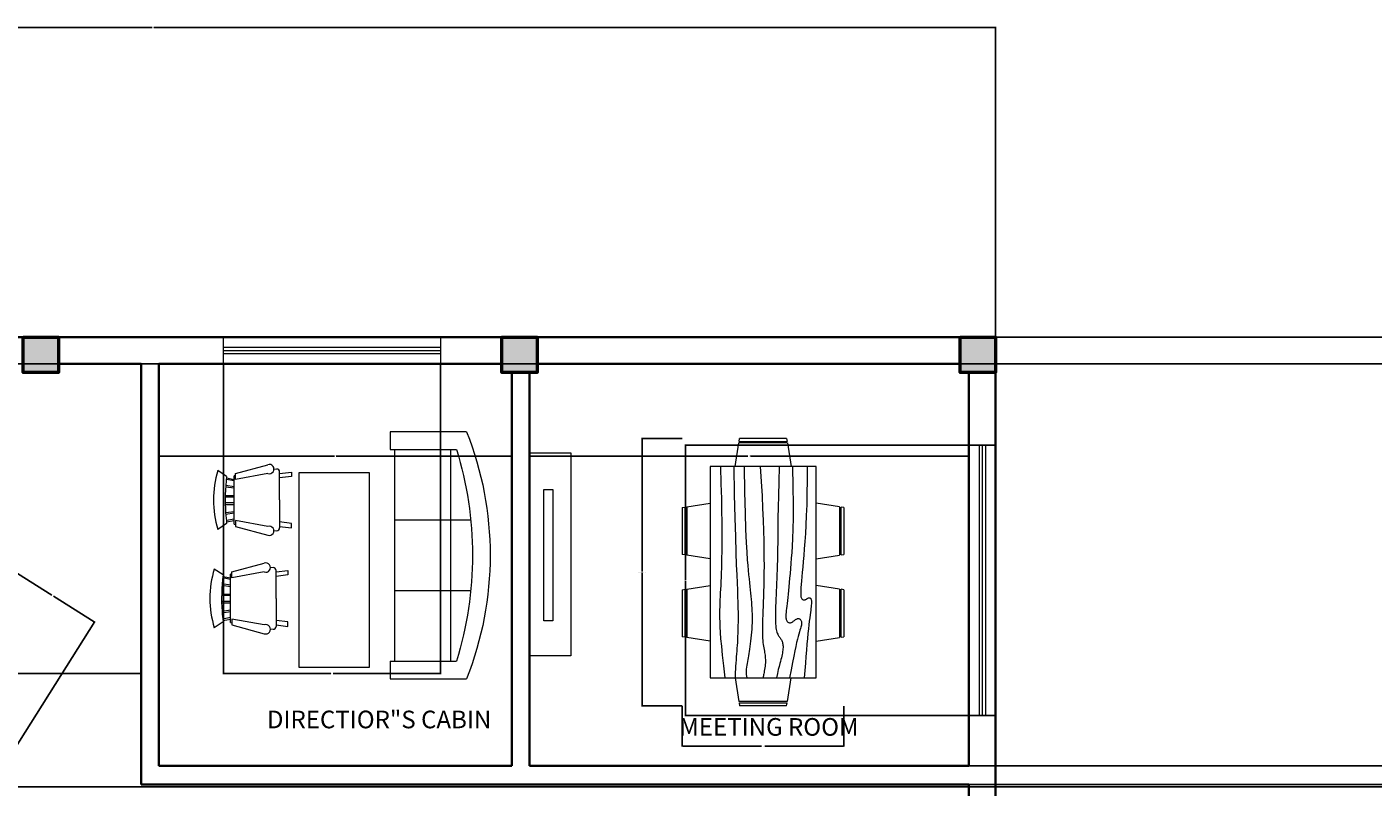
# Model space of a CAD drawing. Units: inches. Extents: x 369 to 4994, y 516 to 1297.
# Tile 6 of 9: x 1452 to 1910, y 886 to 1144. Entities that reach past the tile are written whole.
import ezdxf

# ---------------------------------------------------------------- set-up
doc = ezdxf.new("R2010")
doc.units = ezdxf.units.IN
doc.header["$MEASUREMENT"] = 0
for name, color, linetype, lineweight in [('A-ANNO-DIMS', 2, 'Continuous', 18), ('A-AREA-IDEN', 7, 'Continuous', 18), ('A-COLS', 7, 'Continuous', 50), ('A-FURN', 8, 'Continuous', 18), ('A-GLAZ', 4, 'Continuous', 18), ('A-WALL', 7, 'Continuous', 35)]:
    doc.layers.add(name, color=color, linetype=linetype, lineweight=lineweight)
doc.layers.add('A-COLS-PATT', color=18, linetype='Continuous', lineweight=13, true_color=0x000000)
doc.styles.get("Standard").update_dxf_attribs({"font": 'arial.ttf'})
doc.dimstyles.get("Standard").update_dxf_attribs({"dimtxt": 0.18, "dimasz": 0.18, "dimexe": 0.18, "dimexo": 0.0625, "dimgap": 0.09, "dimtad": 0, "dimtih": 1, "dimtoh": 1, "dimdec": 4, "dimzin": 0, "dimdsep": 46, "dimtxsty": 'Standard', "dimcen": 0.09, "dimadec": 0, "dimazin": 0, "dimtfac": 1, "dimtdec": 4, "dimtofl": 0, "dimtmove": 0, "dimatfit": 3, "dimfxl": 1, "dimtolj": 1, "dimtzin": 0, "dimarcsym": 0})

# ---------------------------------------------------------------- blocks, each defined once
blk = doc.blocks.new('Dining Set - 36 x 72 in.')
for p, q in [((-22, 27.5), (-22.1562, 26.50042)), ((-22, 27.5), (-6, 27.5)), ((-5.8437, 26.49966), (-6, 27.5)), ((6, 27.5), (5.8438, 26.50042)), ((6, 27.5), (22, 27.5)), ((22.1563, 26.49966), (22, 27.5)), ((-22.2343, 26.00059), (-23.4847, 17.99762)), ((-22.2304, 26), (-5.7608, 26)), ((-5.8416, 26.5), (-22.1534, 26.5)), ((-4.5152, 17.99762), (-5.7655, 25.99926)), ((5.7657, 26.00059), (4.5153, 17.99762)), ((5.7696, 26), (22.2392, 26)), ((22.1584, 26.5), (5.8466, 26.5)), ((23.4848, 17.99762), (22.2345, 25.99926)), ((36, 18), (-36, 18)), ((-36, 18), (-36, -18)), ((36, -18), (36, 18)), ((-44.0006, 8.23428), (-35.9976, 9.48474)), ((44.0006, 8.23428), (35.9976, 9.48474)), ((-45.5, 8), (-44.5004, 8.15617)), ((-45.5, 8), (-45.5, -8)), ((-44.5, -8.15843), (-44.5, 8.15338)), ((-44, 8.23041), (-44, -8.23915)), ((44, 8.23041), (44, -8.23915)), ((44.5, -8.15843), (44.5, 8.15338)), ((45.5, 8), (44.5005, 8.15617)), ((45.5, 8), (45.5, -8)), ((-44.4997, -8.15631), (-45.5, -8)), ((-35.9976, -9.48476), (-43.9993, -8.2345)), ((35.9976, -9.48476), (43.9993, -8.2345)), ((44.4997, -8.15631), (45.5, -8)), ((-36, -18), (36, -18)), ((-22.2343, -26.0006), (-23.4847, -17.99762)), ((-4.5152, -17.99762), (-5.7655, -25.99928)), ((5.7657, -26.0006), (4.5153, -17.99762)), ((23.4848, -17.99762), (22.2345, -25.99928)), ((-22.2304, -26), (-5.7608, -26)), ((-22, -27.5), (-22.1562, -26.50044)), ((-5.8416, -26.5), (-22.1534, -26.5)), ((-5.8437, -26.49967), (-6, -27.5)), ((5.7696, -26), (22.2392, -26)), ((6, -27.5), (5.8438, -26.50044)), ((22.1584, -26.5), (5.8466, -26.5)), ((22.1563, -26.49967), (22, -27.5)), ((-22, -27.5), (-6, -27.5)), ((6, -27.5), (22, -27.5))]:
    blk.add_line(p, q)
for points in [[(-36, 15), (-31.1772, 14.97754), (-26.8079, 14.91406), (-22.8538, 14.81543), (-19.276, 14.6875), (-16.0362, 14.53613), (-13.0957, 14.36718), (-10.4159, 14.18652), (-7.9583, 14), (-5.6904, 13.81315), (-3.6035, 13.63021), (-1.6954, 13.45508), (0.0365, 13.29166), (1.5945, 13.14388), (2.9811, 13.01562), (4.1988, 12.9108), (5.25, 12.83333), (6.1393, 12.78613), (6.8802, 12.76823), (7.4883, 12.77767), (7.9792, 12.8125), (8.3685, 12.87077), (8.6719, 12.95052), (8.9049, 13.0498), (9.0833, 13.16666), (9.2205, 13.29899), (9.3216, 13.44401), (9.3895, 13.59879), (9.4271, 13.76041), (9.4373, 13.92594), (9.4232, 14.09245), (9.3875, 14.257), (9.3333, 14.41666), (9.2638, 14.56917), (9.1836, 14.71484), (9.0975, 14.85465), (9.0104, 14.98958), (8.9272, 15.1206), (8.8529, 15.2487), (8.7922, 15.37483), (8.75, 15.5), (8.7305, 15.62467), (8.7344, 15.74739), (8.7617, 15.86621), (8.8125, 15.97916), (8.8867, 16.08431), (8.9844, 16.17968), (9.1055, 16.26334), (9.25, 16.33333), (9.4189, 16.38802), (9.6172, 16.42708), (9.8506, 16.45052), (10.125, 16.45833), (10.4463, 16.45052), (10.8203, 16.42708), (11.2529, 16.38802), (11.75, 16.33333), (12.3184, 16.26318), (12.9694, 16.17838), (13.7151, 16.07991), (14.5677, 15.96875), (15.5395, 15.84586), (16.6426, 15.71224), (17.8893, 15.56884), (19.2917, 15.41666), (20.859, 15.25667), (22.5879, 15.08984), (24.4721, 14.91715), (26.5052, 14.73958), (28.6809, 14.5581), (30.9929, 14.3737), (33.4347, 14.18733), (36, 14)], [(-36, 10), (-28.9766, 10.14274), (-23.1725, 10.20442), (-18.4241, 10.19775), (-14.5677, 10.13541), (-11.4399, 10.03011), (-8.877, 9.89453), (-6.7154, 9.74137), (-4.7917, 9.58333), (-2.9698, 9.43082), (-1.2246, 9.28515), (0.4415, 9.14534), (2.026, 9.01041), (3.5266, 8.87939), (4.9408, 8.7513), (6.266, 8.62516), (7.5, 8.5), (8.6411, 8.37549), (9.6914, 8.2539), (10.6538, 8.13818), (11.5312, 8.03125), (12.3267, 7.93603), (13.043, 7.85547), (13.6831, 7.79248), (14.25, 7.75), (14.7471, 7.7303), (15.1797, 7.73307), (15.5537, 7.75732), (15.875, 7.80208), (16.1494, 7.86637), (16.3828, 7.94922), (16.5811, 8.04964), (16.75, 8.16666), (16.8944, 8.29915), (17.0143, 8.44531), (17.1089, 8.60319), (17.1771, 8.77083), (17.218, 8.94629), (17.2305, 9.1276), (17.2137, 9.31282), (17.1667, 9.5), (17.0895, 9.6875), (16.987, 9.875), (16.8649, 10.0625), (16.7292, 10.25), (16.5856, 10.4375), (16.4401, 10.625), (16.2985, 10.8125), (16.1667, 11), (16.05, 11.18733), (15.9518, 11.3737), (15.8752, 11.5581), (15.8229, 11.73958), (15.798, 11.91715), (15.8034, 12.08984), (15.842, 12.25667), (15.9167, 12.41666), (16.0295, 12.56836), (16.1784, 12.70833), (16.3605, 12.83268), (16.5729, 12.9375), (16.8127, 13.01888), (17.0768, 13.07291), (17.3625, 13.0957), (17.6667, 13.08333), (17.9894, 13.03312), (18.3418, 12.94726), (18.7382, 12.82918), (19.1927, 12.68229), (19.7195, 12.51001), (20.3327, 12.31575), (21.0465, 12.10294), (21.875, 11.875), (22.8357, 11.63354), (23.959, 11.37304), (25.2786, 11.08618), (26.8282, 10.76562), (28.6414, 10.40405), (30.752, 9.99414), (33.1936, 9.52856), (36, 9)], [(-36, 5.5), (-30.7157, 5.3348), (-26.069, 5.20963), (-21.9946, 5.11767), (-18.4271, 5.05208), (-15.3009, 5.00602), (-12.5508, 4.97265), (-10.1112, 4.94515), (-7.9167, 4.91666), (-5.909, 4.88167), (-4.0586, 4.83984), (-2.3429, 4.79215), (-0.7396, 4.73958), (0.7739, 4.6831), (2.22, 4.6237), (3.6213, 4.56233), (5, 4.5), (6.373, 4.43782), (7.7344, 4.3776), (9.0723, 4.32129), (10.375, 4.27083), (11.6309, 4.22819), (12.8281, 4.19531), (13.9551, 4.17415), (15, 4.16666), (15.954, 4.17448), (16.819, 4.19791), (17.6001, 4.23698), (18.3021, 4.29166), (18.9299, 4.36198), (19.4883, 4.44791), (19.9823, 4.54948), (20.4167, 4.66666), (20.7969, 4.79899), (21.1302, 4.94401), (21.4245, 5.09879), (21.6875, 5.26041), (21.9271, 5.42594), (22.1511, 5.59245), (22.3672, 5.757), (22.5834, 5.91666), (22.8065, 6.06868), (23.0404, 6.21093), (23.2879, 6.34147), (23.5521, 6.45833), (23.8358, 6.55957), (24.142, 6.64323), (24.4735, 6.70735), (24.8334, 6.75), (25.2235, 6.76969), (25.642, 6.76692), (26.0858, 6.74267), (26.5521, 6.69791), (27.0379, 6.63362), (27.5404, 6.55078), (28.0565, 6.45036), (28.5834, 6.33333), (29.1242, 6.19987), (29.7071, 6.04687), (30.3661, 5.87044), (31.1354, 5.66666), (32.0493, 5.43164), (33.142, 5.16146), (34.4475, 4.85221), (36, 4.5)], [(-36, -1), (-30.7915, -0.6591), (-26.0195, -0.38216), (-21.6519, -0.16284), (-17.6563, 0.00521), (-14.0005, 0.12833), (-10.6523, 0.21289), (-7.5796, 0.26522), (-4.75, 0.29166), (-2.134, 0.29793), (0.2878, 0.28711), (2.5317, 0.26163), (4.6146, 0.22396), (6.5529, 0.17651), (8.3633, 0.12174), (10.0623, 0.06209), (11.6667, 0), (13.1899, -0.06201), (14.6341, -0.1211), (15.9982, -0.17432), (17.2813, -0.21875), (18.4823, -0.25147), (19.6003, -0.26953), (20.6343, -0.27002), (21.5834, -0.25), (22.4481, -0.20768), (23.2357, -0.14584), (23.9549, -0.06836), (24.6146, 0.02083), (25.2235, 0.11784), (25.7904, 0.21875), (26.3241, 0.31966), (26.8334, 0.41666), (27.3265, 0.50618), (27.8099, 0.58593), (28.2894, 0.65397), (28.7709, 0.70833), (29.2601, 0.74707), (29.763, 0.76823), (30.2855, 0.76985), (30.8334, 0.75), (31.4088, 0.70784), (31.9994, 0.64713), (32.589, 0.57275), (33.1615, 0.48958), (33.7008, 0.4025), (34.1908, 0.3164), (34.6153, 0.23616), (34.9584, 0.16666), (35.2099, 0.11165), (35.3848, 0.07031), (35.504, 0.04069), (35.5886, 0.02083), (35.6594, 0.00879), (35.7377, 0.0026), (35.8442, 0.00032), (36, 0)], [(-36, -6.5), (-27.1843, -6.31267), (-20.084, -6.1263), (-14.469, -5.9419), (-10.1094, -5.76042), (-6.7752, -5.58285), (-4.2363, -5.41016), (-2.2629, -5.24333), (-0.625, -5.08334), (0.8708, -4.93099), (2.2715, -4.78646), (3.5872, -4.64974), (4.8281, -4.52084), (6.0046, -4.39974), (7.127, -4.28646), (8.2053, -4.18099), (9.25, -4.08334), (10.2705, -3.99382), (11.2734, -3.91407), (12.2647, -3.84603), (13.25, -3.79167), (14.2354, -3.75293), (15.2266, -3.73177), (16.2295, -3.73015), (17.25, -3.75), (18.2912, -3.79248), (19.3451, -3.85547), (20.4009, -3.93604), (21.4479, -4.03125), (22.4754, -4.13819), (23.4727, -4.25391), (24.4289, -4.37549), (25.3334, -4.5), (26.1785, -4.62492), (26.9694, -4.74935), (27.7145, -4.87281), (28.4219, -4.99479), (29.1, -5.11483), (29.7572, -5.23242), (30.4016, -5.34709), (31.0417, -5.45834), (31.6837, -5.56437), (32.3262, -5.65821), (32.9658, -5.73153), (33.599, -5.77604), (34.2224, -5.78345), (34.8327, -5.74545), (35.4264, -5.65373), (36, -5.5)], [(-36, -10), (-26.4022, -9.81299), (-18.4675, -9.62891), (-11.9839, -9.45069), (-6.7396, -9.28125), (-2.5226, -9.12354), (0.8789, -8.98047), (3.6769, -8.85498), (6.0833, -8.75), (8.2767, -8.66765), (10.3021, -8.60677), (12.1712, -8.56543), (13.8958, -8.54167), (15.4876, -8.53353), (16.9583, -8.53907), (18.3197, -8.55632), (19.5834, -8.58334), (20.7616, -8.61841), (21.8685, -8.66081), (22.9188, -8.71004), (23.9271, -8.76563), (24.9081, -8.82707), (25.8763, -8.89388), (26.8465, -8.96558), (27.8334, -9.04167), (28.8474, -9.12118), (29.8828, -9.20117), (30.93, -9.27824), (31.9792, -9.34896), (33.0205, -9.40991), (34.0443, -9.45768), (35.0407, -9.48885), (36, -9.5)], [(-36, -14.5), (-30.0881, -14.33513), (-25.0332, -14.21224), (-20.7312, -14.12647), (-17.0781, -14.07292), (-13.97, -14.04671), (-11.3027, -14.04297), (-8.9724, -14.05681), (-6.875, -14.08334), (-4.9224, -14.11833), (-3.0905, -14.16016), (-1.3709, -14.20785), (0.2448, -14.26042), (1.7647, -14.3169), (3.1973, -14.3763), (4.5507, -14.43767), (5.8333, -14.5), (7.0554, -14.5621), (8.235, -14.62175), (9.3922, -14.67652), (10.5469, -14.72396), (11.7192, -14.76164), (12.929, -14.78711), (14.1965, -14.79794), (15.5417, -14.79167), (16.9933, -14.76424), (18.6152, -14.70508), (20.4804, -14.60197), (22.6615, -14.44271), (25.2312, -14.21509), (28.2624, -13.9069), (31.8277, -13.50594), (36, -13)]]:
    blk.add_lwpolyline(points)
blk = doc.blocks.new('Chair - Rocking')
for p, q in [((-8, -4.5), (-10, -1.5)), ((-7.5, -4.5), (-7, -7)), ((-6.5, -7), (-7.02225, -4.43)), ((-4.5, -7), (-4.96674, -4.19951)), ((-4, -7), (-4.40532, -4.16272)), ((-1.5, -4.05012), (-1.5, -7)), ((-1, -7), (-1, -4.05012)), ((1, -7), (1, -4.04655)), ((1.5, -4.05012), (1.5, -7)), ((4, -7), (4.40187, -4.18694)), ((4.5, -7), (4.96761, -4.19437)), ((6.5, -7), (7, -4.4057)), ((7.5, -4.5), (7, -7)), ((8, -4.5), (10, -1.5)), ((-9, -7.5), (-12, -18.49999)), ((-7, -7.5), (-9, -7.5)), ((-9, -18.49999), (-7, -7.5)), ((-8.23428, -6.99939), (-8.3093, -7.47958)), ((-8.23041, -7), (8.23915, -7)), ((7, -7.5), (9, -7.5)), ((9, -18.49999), (7, -7.5)), ((8.31071, -7.48854), (8.23449, -7.00073)), ((9, -7.5), (12, -18.49999)), ((-10.36644, -20.64523), (-10.5, -21.49999)), ((-9, -22.49999), (-9.5, -26.49999)), ((0, -22.49999), (-9.5, -22.49999)), ((-8, -26.49999), (-7.5, -22.49999)), ((0, -22.49999), (9.5, -22.49999)), ((8, -26.49999), (7.5, -22.49999)), ((9, -22.49999), (9.5, -26.49999)), ((10.5, -21.49999), (10.3575, -20.58798)), ((-9.5, -26.49999), (-8, -26.49999)), ((9.5, -26.49999), (8, -26.49999))]:
    blk.add_line(p, q)
for centre, radius, start, end in [((0, -34.08333), 34.08333, 72.93847, 107.0615), ((0, -68.25004), 64.25, 93.92211, 97.15267), ((0, -68.25004), 64.25, 82.84733, 93.92211), ((-10.5, -18.99999), 1.58114, 161.5651, 18.43495), ((-9.5, -21.49999), 1, 180, 270), ((10.5, -18.99999), 1.58114, 161.5651, 18.43495), ((9.5, -21.49999), 1, 270, 0)]:
    blk.add_arc(centre, radius, start, end)
blk = doc.blocks.new('Sofa - Roundback 7 ft.')
for p, q in [((-12.00002, -32.4421), (-12.00003, -6.5971)), ((11.99997, -32.4421), (11.99998, -6.5971)), ((-36.000027, -34), (-36.000027, -11.4696)), ((-35.999844, -13.3819), (35.9998, -13.3819)), ((35.99998, -34), (35.99998, -11.4696)), ((-36.000027, -32.4421), (35.99998, -32.4421))]:
    blk.add_line(p, q)
for points in [[(-36.000027, -34), (-42.000027, -34), (-42.000027, -8)], [(41.99998, -8), (41.99998, -34), (35.99998, -34)]]:
    blk.add_lwpolyline(points)
for centre, radius, start, end in [((0, -114.25), 114.25, 68.43141, 111.5686), ((-0.00001, -127.1968), 121.1968, 72.72033, 107.2797)]:
    blk.add_arc(centre, radius, start, end)
blk = doc.blocks.new('*D17')
at = {"layer": 'A-ANNO-DIMS', "color": 0, "lineweight": -2, "transparency": 16777216}
for p, q in [((1674.81, 1004.36), (1661.04, 1004.36)), ((1661.22, 1004.18), (1661.22, 959.05)), ((1661.22, 913.54), (1661.22, 958.68)), ((1674.81, 913.36), (1661.04, 913.36))]:
    blk.add_line(p, q, dxfattribs=at)
at = {"layer": 'A-ANNO-DIMS', "color": 0, "transparency": 16777216}
for points in [[(1661.19, 1004.18), (1661.25, 1004.18), (1661.22, 1004.36)], [(1661.19, 913.54), (1661.25, 913.54), (1661.22, 913.36)]]:
    blk.add_solid(points, dxfattribs=at)
at = {"layer": 'Defpoints', "color": 0, "transparency": 16777216}
for p in [(1674.87, 1004.36), (1661.22, 913.36), (1674.87, 913.36)]:
    blk.add_point(p, dxfattribs=at)
at = {"layer": 'A-ANNO-DIMS', "color": 0, "transparency": 16777216, "insert": (1661.22, 958.86), "char_height": 0.18, "attachment_point": 5}
blk.add_mtext('\\A1;TABLE & CHAIRS 91 TYP.', dxfattribs=at)
blk = doc.blocks.new('*D18')
at = {"layer": 'A-ANNO-DIMS', "color": 0, "lineweight": -2, "transparency": 16777216}
for p, q in [((1674.87, 913.3), (1674.87, 899.53)), ((1729.87, 913.3), (1729.87, 899.53)), ((1675.05, 899.71), (1701.84, 899.71)), ((1729.69, 899.71), (1702.9, 899.71))]:
    blk.add_line(p, q, dxfattribs=at)
at = {"layer": 'A-ANNO-DIMS', "color": 0, "transparency": 16777216}
for points in [[(1675.05, 899.74), (1675.05, 899.68), (1674.87, 899.71)], [(1729.69, 899.74), (1729.69, 899.68), (1729.87, 899.71)]]:
    blk.add_solid(points, dxfattribs=at)
at = {"layer": 'Defpoints', "color": 0, "transparency": 16777216}
for p in [(1674.87, 913.36), (1729.87, 913.36), (1729.87, 899.71)]:
    blk.add_point(p, dxfattribs=at)
at = {"layer": 'A-ANNO-DIMS', "color": 0, "transparency": 16777216, "insert": (1702.37, 899.71), "char_height": 0.18, "attachment_point": 5}
blk.add_mtext('\\A1;55 TYP.', dxfattribs=at)
blk = doc.blocks.new('*D46')
at = {"layer": 'A-ANNO-DIMS', "color": 0, "lineweight": -2, "transparency": 16777216}
for p, q in [((978.32, 1029.79), (2671.51, 1029.79)), ((2671.33, 1029.61), (2671.33, 957.97)), ((2671.33, 885.97), (2671.33, 957.61)), ((1038.32, 885.79), (2671.51, 885.79))]:
    blk.add_line(p, q, dxfattribs=at)
at = {"layer": 'A-ANNO-DIMS', "color": 0, "transparency": 16777216}
for points in [[(2671.3, 1029.61), (2671.36, 1029.61), (2671.33, 1029.79)], [(2671.3, 885.97), (2671.36, 885.97), (2671.33, 885.79)]]:
    blk.add_solid(points, dxfattribs=at)
at = {"layer": 'Defpoints', "color": 0, "transparency": 16777216}
for p in [(978.26, 1029.79), (2671.33, 1029.79), (1038.26, 885.79)]:
    blk.add_point(p, dxfattribs=at)
at = {"layer": 'A-ANNO-DIMS', "color": 0, "transparency": 16777216, "insert": (2671.33, 957.79), "char_height": 0.18, "attachment_point": 5}
blk.add_mtext('\\A1;144', dxfattribs=at)
blk = doc.blocks.new('*D74')
at = {"layer": 'A-ANNO-DIMS', "color": 0, "lineweight": -2, "transparency": 16777216}
for p, q in [((1208.37, 1038.85), (1208.37, 1144.37)), ((1208.55, 1144.19), (1494.58, 1144.19)), ((1781.19, 1144.19), (1495.16, 1144.19)), ((1781.37, 1038.85), (1781.37, 1144.37))]:
    blk.add_line(p, q, dxfattribs=at)
at = {"layer": 'A-ANNO-DIMS', "color": 0, "transparency": 16777216}
for points in [[(1208.55, 1144.22), (1208.55, 1144.16), (1208.37, 1144.19)], [(1781.19, 1144.22), (1781.19, 1144.16), (1781.37, 1144.19)]]:
    blk.add_solid(points, dxfattribs=at)
at = {"layer": 'Defpoints', "color": 0, "transparency": 16777216}
for p in [(1781.37, 1144.19), (1208.37, 1038.79), (1781.37, 1038.79)]:
    blk.add_point(p, dxfattribs=at)
at = {"layer": 'A-ANNO-DIMS', "color": 0, "transparency": 16777216, "insert": (1494.87, 1144.19), "char_height": 0.18, "attachment_point": 5}
blk.add_mtext('\\A1;573', dxfattribs=at)
blk = doc.blocks.new('*D76')
at = {"layer": 'A-ANNO-DIMS', "color": 0, "lineweight": -2, "transparency": 16777216}
for p, q in [((1277.37, 1029.73), (1277.37, 924.21)), ((1490.89, 1029.73), (1490.89, 924.21)), ((1277.55, 924.39), (1383.74, 924.39)), ((1490.71, 924.39), (1384.53, 924.39))]:
    blk.add_line(p, q, dxfattribs=at)
at = {"layer": 'A-ANNO-DIMS', "color": 0, "transparency": 16777216}
for points in [[(1277.55, 924.42), (1277.55, 924.36), (1277.37, 924.39)], [(1490.71, 924.42), (1490.71, 924.36), (1490.89, 924.39)]]:
    blk.add_solid(points, dxfattribs=at)
at = {"layer": 'Defpoints', "color": 0, "transparency": 16777216}
for p in [(1277.37, 1029.79), (1490.89, 1029.79), (1277.37, 924.39)]:
    blk.add_point(p, dxfattribs=at)
at = {"layer": 'A-ANNO-DIMS', "color": 0, "transparency": 16777216, "insert": (1384.13, 924.39), "char_height": 0.18, "attachment_point": 5}
blk.add_mtext('\\A1;213.5', dxfattribs=at)
blk = doc.blocks.new('*D77')
at = {"layer": 'A-ANNO-DIMS', "color": 0, "lineweight": -2, "transparency": 16777216}
for p, q in [((1496.89, 893.03), (1496.89, 998.55)), ((1497.07, 998.37), (1556.61, 998.37)), ((1616.71, 998.37), (1557.17, 998.37)), ((1616.89, 893.03), (1616.89, 998.55))]:
    blk.add_line(p, q, dxfattribs=at)
at = {"layer": 'A-ANNO-DIMS', "color": 0, "transparency": 16777216}
for points in [[(1497.07, 998.4), (1497.07, 998.34), (1496.89, 998.37)], [(1616.71, 998.4), (1616.71, 998.34), (1616.89, 998.37)]]:
    blk.add_solid(points, dxfattribs=at)
at = {"layer": 'Defpoints', "color": 0, "transparency": 16777216}
for p in [(1616.89, 998.37), (1496.89, 892.97), (1616.89, 892.97)]:
    blk.add_point(p, dxfattribs=at)
at = {"layer": 'A-ANNO-DIMS', "color": 0, "transparency": 16777216, "insert": (1556.89, 998.37), "char_height": 0.18, "attachment_point": 5}
blk.add_mtext('\\A1;120', dxfattribs=at)
blk = doc.blocks.new('*D78')
at = {"layer": 'A-ANNO-DIMS', "color": 0, "lineweight": -2, "transparency": 16777216}
for p, q in [((1622.89, 893.03), (1622.89, 998.55)), ((1623.07, 998.37), (1697.18, 998.37)), ((1772.19, 998.37), (1698.09, 998.37)), ((1772.37, 893.03), (1772.37, 998.55))]:
    blk.add_line(p, q, dxfattribs=at)
at = {"layer": 'A-ANNO-DIMS', "color": 0, "transparency": 16777216}
for points in [[(1623.07, 998.4), (1623.07, 998.34), (1622.89, 998.37)], [(1772.19, 998.4), (1772.19, 998.34), (1772.37, 998.37)]]:
    blk.add_solid(points, dxfattribs=at)
at = {"layer": 'Defpoints', "color": 0, "transparency": 16777216}
for p in [(1772.37, 998.37), (1622.89, 892.97), (1772.37, 892.97)]:
    blk.add_point(p, dxfattribs=at)
at = {"layer": 'A-ANNO-DIMS', "color": 0, "transparency": 16777216, "insert": (1697.63, 998.37), "char_height": 0.18, "attachment_point": 5}
blk.add_mtext('\\A1;149.48', dxfattribs=at)
blk = doc.blocks.new('*D79')
at = {"layer": 'A-ANNO-DIMS', "color": 0, "lineweight": -2, "transparency": 16777216}
for p, q in [((1769.44, 1029.79), (2671.51, 1029.79)), ((2671.33, 1029.61), (2671.33, 961.56)), ((2671.33, 893.15), (2671.33, 961.2)), ((1772.44, 892.97), (2671.51, 892.97))]:
    blk.add_line(p, q, dxfattribs=at)
at = {"layer": 'A-ANNO-DIMS', "color": 0, "transparency": 16777216}
for points in [[(2671.3, 1029.61), (2671.36, 1029.61), (2671.33, 1029.79)], [(2671.3, 893.15), (2671.36, 893.15), (2671.33, 892.97)]]:
    blk.add_solid(points, dxfattribs=at)
at = {"layer": 'Defpoints', "color": 0, "transparency": 16777216}
for p in [(1769.37, 1029.79), (2671.33, 1029.79), (1772.37, 892.97)]:
    blk.add_point(p, dxfattribs=at)
at = {"layer": 'A-ANNO-DIMS', "color": 0, "transparency": 16777216, "insert": (2671.33, 961.38), "char_height": 0.18, "attachment_point": 5}
blk.add_mtext('\\A1;136.82', dxfattribs=at)
blk = doc.blocks.new('*D80')
at = {"layer": 'A-ANNO-DIMS', "color": 0, "lineweight": -2, "transparency": 16777216}
for p, q in [((1772.44, 886.6), (2671.51, 886.6)), ((2671.33, 886.42), (2671.33, 847.38)), ((2671.33, 807.97), (2671.33, 847.01)), ((1772.44, 807.79), (2671.51, 807.79))]:
    blk.add_line(p, q, dxfattribs=at)
at = {"layer": 'A-ANNO-DIMS', "color": 0, "transparency": 16777216}
for points in [[(2671.3, 886.42), (2671.36, 886.42), (2671.33, 886.6)], [(2671.3, 807.97), (2671.36, 807.97), (2671.33, 807.79)]]:
    blk.add_solid(points, dxfattribs=at)
at = {"layer": 'Defpoints', "color": 0, "transparency": 16777216}
for p in [(1772.37, 886.6), (2671.33, 886.6), (1772.37, 807.79)]:
    blk.add_point(p, dxfattribs=at)
at = {"layer": 'A-ANNO-DIMS', "color": 0, "transparency": 16777216, "insert": (2671.33, 847.19), "char_height": 0.18, "attachment_point": 5}
blk.add_mtext('\\A1;78.81', dxfattribs=at)
blk = doc.blocks.new('*D88')
at = {"layer": 'A-ANNO-DIMS', "color": 0, "lineweight": -2, "transparency": 16777216}
for p, q in [((1390.27, 870.84), (1446.63, 960.04)), ((1446.68, 959.8), (1460.49, 951.07)), ((1474.87, 941.99), (1461.06, 950.71)), ((1418.75, 852.84), (1475.12, 942.04))]:
    blk.add_line(p, q, dxfattribs=at)
at = {"layer": 'A-ANNO-DIMS', "color": 0, "transparency": 16777216}
for points in [[(1446.7, 959.82), (1446.67, 959.77), (1446.53, 959.89)], [(1474.88, 942.01), (1474.85, 941.96), (1475.02, 941.89)]]:
    blk.add_solid(points, dxfattribs=at)
at = {"layer": 'Defpoints', "color": 0, "transparency": 16777216}
for p in [(1475.02, 941.89), (1390.23, 870.79), (1418.72, 852.79)]:
    blk.add_point(p, dxfattribs=at)
at = {"layer": 'A-ANNO-DIMS', "color": 0, "transparency": 16777216, "insert": (1460.78, 950.89), "char_height": 0.18, "attachment_point": 5}
blk.add_mtext('\\A1;33.7', dxfattribs=at)
blk = doc.blocks.new('*D94')
at = {"layer": 'A-ANNO-DIMS', "color": 0, "lineweight": -2, "transparency": 16777216}
for p, q in [((1518.87, 1029.73), (1518.87, 924.21)), ((1592.65, 1029.73), (1592.65, 924.21)), ((1519.05, 924.39), (1555.37, 924.39)), ((1592.47, 924.39), (1556.15, 924.39))]:
    blk.add_line(p, q, dxfattribs=at)
at = {"layer": 'A-ANNO-DIMS', "color": 0, "transparency": 16777216}
for points in [[(1519.05, 924.42), (1519.05, 924.36), (1518.87, 924.39)], [(1592.47, 924.42), (1592.47, 924.36), (1592.65, 924.39)]]:
    blk.add_solid(points, dxfattribs=at)
at = {"layer": 'Defpoints', "color": 0, "transparency": 16777216}
for p in [(1518.87, 1029.79), (1592.65, 1029.79), (1518.87, 924.39)]:
    blk.add_point(p, dxfattribs=at)
at = {"layer": 'A-ANNO-DIMS', "color": 0, "transparency": 16777216, "insert": (1555.76, 924.39), "char_height": 0.18, "attachment_point": 5}
blk.add_mtext('\\A1;73.77', dxfattribs=at)
blk = doc.blocks.new('*D95')
at = {"layer": 'A-ANNO-DIMS', "color": 0, "lineweight": -2, "transparency": 16777216}
for p, q in [((1781.31, 1002.1), (1675.79, 1002.1)), ((1675.97, 1001.92), (1675.97, 956.27)), ((1675.97, 910.26), (1675.97, 955.91)), ((1781.31, 910.08), (1675.79, 910.08))]:
    blk.add_line(p, q, dxfattribs=at)
at = {"layer": 'A-ANNO-DIMS', "color": 0, "transparency": 16777216}
for points in [[(1675.94, 1001.92), (1676, 1001.92), (1675.97, 1002.1)], [(1675.94, 910.26), (1676, 910.26), (1675.97, 910.08)]]:
    blk.add_solid(points, dxfattribs=at)
at = {"layer": 'Defpoints', "color": 0, "transparency": 16777216}
for p in [(1675.97, 1002.1), (1781.37, 1002.1), (1781.37, 910.08)]:
    blk.add_point(p, dxfattribs=at)
at = {"layer": 'A-ANNO-DIMS', "color": 0, "transparency": 16777216, "insert": (1675.97, 956.09), "char_height": 0.18, "attachment_point": 5}
blk.add_mtext('\\A1;92.02', dxfattribs=at)
blk = doc.blocks.new('*D98')
at = {"layer": 'A-ANNO-DIMS', "color": 0, "lineweight": -2, "transparency": 16777216}
for p, q in [((1992.86, 1038.79), (368.68, 1038.79)), ((368.86, 1038.61), (368.86, 830.47)), ((368.86, 621.97), (368.86, 830.11)), ((2046.86, 621.79), (368.68, 621.79))]:
    blk.add_line(p, q, dxfattribs=at)
at = {"layer": 'A-ANNO-DIMS', "color": 0, "transparency": 16777216}
for points in [[(368.83, 1038.61), (368.89, 1038.61), (368.86, 1038.79)], [(368.83, 621.97), (368.89, 621.97), (368.86, 621.79)]]:
    blk.add_solid(points, dxfattribs=at)
at = {"layer": 'Defpoints', "color": 0, "transparency": 16777216}
for p in [(368.86, 1038.79), (1992.93, 1038.79), (2046.93, 621.79)]:
    blk.add_point(p, dxfattribs=at)
at = {"layer": 'A-ANNO-DIMS', "color": 0, "transparency": 16777216, "insert": (368.86, 830.29), "char_height": 0.18, "attachment_point": 5}
blk.add_mtext('\\A1;417', dxfattribs=at)

msp = doc.modelspace()

# ---------------------------------------------------------------- hatches: boundary and pattern name
at = {"layer": 'A-COLS-PATT'}
h = msp.add_hatch(color=256, dxfattribs=at)
h.dxf.hatch_style = 1
h.paths.add_polyline_path([(540.2581, 633.7894), (528.2581, 633.7894), (528.2581, 621.7894), (540.2581, 621.7894)])
h.paths.add_polyline_path([(726.2581, 633.7894), (714.2581, 633.7894), (714.2581, 621.7894), (726.2581, 621.7894)])
h.paths.add_polyline_path([(918.2581, 633.7894), (906.2581, 633.7894), (906.2581, 621.7894), (918.2581, 621.7894)])
h.paths.add_polyline_path([(1047.2581, 633.7894), (1035.2581, 633.7894), (1035.2581, 621.7894), (1047.2581, 621.7894)])
h.paths.add_polyline_path([(1047.2581, 798.6977), (1035.2581, 798.6977), (1035.2581, 786.6977), (1047.2581, 786.6977)])
h.paths.add_polyline_path([(918.2581, 795.7894), (906.2581, 795.7894), (906.2581, 783.7894), (918.2581, 783.7894)])
h.paths.add_polyline_path([(726.2581, 795.7894), (714.2581, 795.7894), (714.2581, 783.7894), (726.2581, 783.7894)])
h.paths.add_polyline_path([(1047.2581, 1038.7894), (1035.2581, 1038.7894), (1035.2581, 1026.7894), (1047.2581, 1026.7894)])
h.paths.add_polyline_path([(855.044, 1038.7894), (843.044, 1038.7894), (843.044, 1026.7894), (855.044, 1026.7894)])
h.paths.add_polyline_path([(728.5536, 1038.7894), (716.5536, 1038.7894), (716.5536, 1026.7894), (728.5536, 1026.7894)])
h.paths.add_polyline_path([(543.2581, 1038.7894), (531.2581, 1038.7894), (531.2581, 1026.7894), (543.2581, 1026.7894)])
h.paths.add_polyline_path([(543.2581, 792.9013), (531.2581, 792.9013), (531.2581, 780.9013), (543.2581, 780.9013), (543.2581, 783.7894)])
h.paths.add_polyline_path([(1274.3738, 633.7894), (1262.3738, 633.7894), (1262.3738, 621.7894), (1274.3738, 621.7894)])
h.paths.add_polyline_path([(1460.3738, 633.7894), (1448.3738, 633.7894), (1448.3738, 621.7894), (1460.3738, 621.7894)])
h.paths.add_polyline_path([(1652.3738, 633.7894), (1640.3738, 633.7894), (1640.3738, 621.7894), (1652.3738, 621.7894)])
h.paths.add_polyline_path([(1781.3738, 633.7894), (1769.3738, 633.7894), (1769.3738, 621.7894), (1781.3738, 621.7894)])
h.paths.add_polyline_path([(1781.3738, 1038.7894), (1769.3738, 1038.7894), (1769.3738, 1026.7894), (1781.3738, 1026.7894)])
h.paths.add_polyline_path([(1625.484, 1038.7894), (1613.484, 1038.7894), (1613.484, 1026.7894), (1615.6962, 1026.7894), (1625.484, 1026.7894)])
h.paths.add_polyline_path([(1462.6692, 1038.7894), (1450.6692, 1038.7894), (1450.6692, 1026.7894), (1462.6692, 1026.7894)])
h.paths.add_polyline_path([(1277.3738, 1038.7894), (1265.3738, 1038.7894), (1265.3738, 1026.7894), (1277.3738, 1026.7894)])
h.paths.add_polyline_path([(1460.3738, 807.7894), (1448.3738, 807.7894), (1448.3738, 795.7894), (1460.3738, 795.7894)])
h.paths.add_polyline_path([(1652.3738, 807.7894), (1640.3738, 807.7894), (1640.3738, 795.7894), (1652.3738, 795.7894)])
h.paths.add_polyline_path([(2244.9265, 633.7894), (2232.9265, 633.7894), (2232.9265, 621.7894), (2244.9265, 621.7894)])
h.paths.add_polyline_path([(2058.9265, 633.7894), (2046.9265, 633.7894), (2046.9265, 621.7894), (2058.9265, 621.7894)])
h.paths.add_polyline_path([(2436.9265, 633.7894), (2424.9265, 633.7894), (2424.9265, 621.7894), (2436.9265, 621.7894)])
h.paths.add_polyline_path([(2565.9265, 633.7894), (2553.9265, 633.7894), (2553.9265, 621.7894), (2565.9265, 621.7894)])
h.paths.add_polyline_path([(2565.9265, 798.6977), (2553.9265, 798.6977), (2553.9265, 786.6977), (2565.9265, 786.6977)])
h.paths.add_polyline_path([(2565.9265, 1038.7894), (2553.9265, 1038.7894), (2553.9265, 1026.7894), (2565.9265, 1026.7894)])
h.paths.add_polyline_path([(2436.9265, 1038.7894), (2424.9265, 1038.7894), (2424.9265, 1026.7894), (2436.9265, 1026.7894)])
h.paths.add_polyline_path([(2247.222, 1038.7894), (2235.222, 1038.7894), (2235.222, 1026.7894), (2247.222, 1026.7894)])
h.paths.add_polyline_path([(2061.9265, 1038.7894), (2049.9265, 1038.7894), (2049.9265, 1026.7894), (2061.9265, 1026.7894)])

# ---------------------------------------------------------------- linework, layer by layer
at = {"layer": 'A-COLS'}
for points in [[(1450.6692, 1038.7894), (1462.6692, 1038.7894), (1462.6692, 1026.7894), (1450.6692, 1026.7894)], [(1769.3738, 1038.7894), (1781.3738, 1038.7894), (1781.3738, 1026.7894), (1769.3738, 1026.7894)]]:
    msp.add_lwpolyline(points, close=True, dxfattribs=at)
msp.add_lwpolyline([(1615.6962, 1026.7894), (1613.484, 1026.7894), (1613.484, 1038.7894), (1625.484, 1038.7894), (1625.484, 1026.7894), (1613.484, 1026.7894)], dxfattribs=at)
at = {"layer": 'A-FURN'}
for points in [[(1622.89, 999.4915), (1636.9443, 999.4915), (1636.9443, 930.4139), (1622.89, 930.4139)], [(1544.5252, 992.771), (1568.3867, 992.771), (1568.3867, 926.4443), (1544.5252, 926.4443)], [(1627.7669, 986.9598), (1630.826, 986.9598), (1630.826, 942.3344), (1627.7669, 942.3344)]]:
    msp.add_lwpolyline(points, close=True, dxfattribs=at)
at = {"layer": 'A-GLAZ'}
for p, q in [((1518.8738, 1035.3655), (1592.6464, 1035.3655)), ((1518.8738, 1034.2894), (1592.6464, 1034.2894)), ((1518.8738, 1033.2133), (1592.6464, 1033.2133)), ((1775.7977, 1002.1036), (1775.7977, 910.0819)), ((1776.8738, 1002.1036), (1776.8738, 910.0819)), ((1777.9499, 1002.1036), (1777.9499, 910.0819))]:
    msp.add_line(p, q, dxfattribs=at)
for points in [[(1518.8738, 1038.7894), (1592.6464, 1038.7894), (1592.6464, 1029.7894), (1518.8738, 1029.7894)], [(1781.3738, 1002.1036), (1772.3738, 1002.1036), (1772.3738, 910.0819), (1781.3738, 910.0819)]]:
    msp.add_lwpolyline(points, close=True, dxfattribs=at)
at = {"layer": 'A-WALL'}
for p, q in [((1772.3738, 1038.7894), (1265.3738, 1038.7894)), ((1490.89, 1029.7894), (1462.6692, 1029.7894)), ((1490.89, 886.5988), (1490.89, 1029.7894)), ((1577.1597, 1029.7894), (1496.89, 1029.7894)), ((1496.89, 892.9667), (1496.89, 1029.7894)), ((1544.3738, 1029.7894), (1496.89, 1029.7894)), ((1613.484, 1029.7894), (1496.89, 1029.7894)), ((1616.89, 892.9667), (1616.89, 1026.7894)), ((1622.89, 892.9667), (1622.89, 1026.7894)), ((1769.3738, 1029.7894), (1625.484, 1029.7894)), ((1769.3738, 1029.7894), (1676.3738, 1029.7894)), ((1769.3738, 1029.7894), (1712.3738, 1029.7894)), ((1772.3738, 892.9667), (1772.3738, 1026.7894)), ((1781.3738, 621.7894), (1781.3738, 1029.7894)), ((1616.89, 892.9667), (1496.89, 892.9667)), ((1616.89, 892.9667), (1550.3738, 892.9667)), ((1772.3738, 892.9667), (1622.89, 892.9667)), ((1670.3738, 892.9667), (1622.89, 892.9667)), ((1772.3738, 892.9667), (1676.3738, 892.9667)), ((1772.3738, 886.5988), (1490.89, 886.5988)), ((1772.3738, 732.5675), (1772.3738, 886.5988))]:
    msp.add_line(p, q, dxfattribs=at)

# ---------------------------------------------------------------- block references
at = {"layer": 'A-FURN', "xscale": -1, "rotation": 270}
msp.add_blockref('Sofa - Roundback 7 ft.', (1609.5155, 964.6229), dxfattribs=at)
at = {"layer": 'A-FURN'}
for name, p, rotation in [('Dining Set - 36 x 72 in.', (1702.371, 958.8646), 270), ('Chair - Rocking', (1515.4143, 983.429), 89.99999999999984), ('Chair - Rocking', (1514.1997, 949.9179), 89.99999999999984)]:
    msp.add_blockref(name, p, dxfattribs=dict(at, rotation=rotation))

# ---------------------------------------------------------------- texts
at = {"layer": 'A-AREA-IDEN'}
for s, p in [('DIRECTIOR"S CABIN', (1533.5975, 905.74)), ('MEETING ROOM', (1673.8552, 903.2134))]:
    msp.add_text(s, height=6, dxfattribs=at).set_placement(p)

# ---------------------------------------------------------------- dimensions: what is measured, and where the dimension line sits
at = {"layer": 'A-ANNO-DIMS'}
dim = msp.add_linear_dim(base=(1781.3738, 1144.1894), p1=(1208.3738, 1038.7894), p2=(1781.3738, 1038.7894), dimstyle='Standard', override={"dimdec": 0, "dimlfac": 1, "dimrnd": 0, "dimzin": 0, "dimdsep": 46, "dimlunit": 2}, dxfattribs=at)
dim.commit()
dim.dimension.update_dxf_attribs({"geometry": '*D74', "text_midpoint": (1494.8738, 1144.1894)})
for base, p1, p2, angle, override, picture, middle in [((368.8581, 1038.7894), (2046.9265, 621.7894), (1992.9265, 1038.7894), 90, {"dimdec": 0, "dimlfac": 1, "dimrnd": 0, "dimzin": 0, "dimdsep": 46, "dimlunit": 2}, '*D98', (368.8581, 830.2894)), ((2671.3265, 1029.7894), (1038.2581, 885.7894), (978.2581, 1029.7894), 90, {"dimdec": 0, "dimlfac": 1, "dimrnd": 0, "dimzin": 0, "dimdsep": 46, "dimlunit": 2}, '*D46', (2671.3265, 957.7894)), ((1277.3738, 924.3894), (1490.89, 1029.7894), (1277.3738, 1029.7894), 180, {"dimdec": 1, "dimlfac": 1, "dimrnd": 0, "dimzin": 0, "dimdsep": 46, "dimlunit": 2}, '*D76', (1384.1319, 924.3894)), ((1518.8738, 924.3894), (1592.6464, 1029.7894), (1518.8738, 1029.7894), 180, {"dimdec": 2, "dimlfac": 1, "dimrnd": 0, "dimzin": 0, "dimdsep": 46, "dimlunit": 2}, '*D94', (1555.7601, 924.3894)), ((2671.3265, 1029.7894), (1772.3738, 892.9667), (1769.3738, 1029.7894), 90, {"dimdec": 2, "dimlfac": 1, "dimrnd": 0, "dimzin": 0, "dimdsep": 46, "dimlunit": 2}, '*D79', (2671.3265, 961.378)), ((1616.89, 998.3667), (1496.89, 892.9667), (1616.89, 892.9667), 0, {"dimdec": 0, "dimlfac": 1, "dimrnd": 0, "dimzin": 0, "dimdsep": 46, "dimlunit": 2}, '*D77', (1556.89, 998.3667)), ((1772.3738, 998.3667), (1622.89, 892.9667), (1772.3738, 892.9667), 0, {"dimdec": 2, "dimlfac": 1, "dimrnd": 0, "dimzin": 0, "dimdsep": 46, "dimlunit": 2}, '*D78', (1697.6319, 998.3667)), ((1675.9738, 1002.1036), (1781.3738, 910.0819), (1781.3738, 1002.1036), 90, {"dimdec": 2, "dimlfac": 1, "dimrnd": 0, "dimzin": 0, "dimdsep": 46, "dimlunit": 2}, '*D95', (1675.9738, 956.0927)), ((1475.0201, 941.8927), (1390.232, 870.7894), (1418.7195, 852.7894), 327.712989, {"dimdec": 1, "dimlfac": 1, "dimrnd": 0, "dimzin": 0, "dimdsep": 46, "dimlunit": 2}, '*D88', (1460.7763, 950.8927)), ((2671.3265, 886.5988), (1772.3738, 807.7894), (1772.3738, 886.5988), 90, {"dimdec": 2, "dimlfac": 1, "dimrnd": 0, "dimzin": 0, "dimdsep": 46, "dimlunit": 2}, '*D80', (2671.3265, 847.1941))]:
    dim = msp.add_linear_dim(base=base, p1=p1, p2=p2, angle=angle, dimstyle='Standard', override=override, dxfattribs=at)
    dim.commit()
    dim.dimension.update_dxf_attribs({"geometry": picture, "text_midpoint": middle})
dim = msp.add_linear_dim(base=(1661.221, 913.3646), p1=(1674.871, 1004.3646), p2=(1674.871, 913.3646), angle=270, text='TABLE & CHAIRS <> TYP.', dimstyle='Standard', override={"dimdec": 0, "dimlfac": 1, "dimrnd": 0, "dimzin": 0, "dimdsep": 46, "dimlunit": 2}, dxfattribs=at)
dim.commit()
dim.dimension.update_dxf_attribs({"geometry": '*D17', "text_midpoint": (1661.221, 958.8646)})
dim = msp.add_linear_dim(base=(1729.871, 899.7146), p1=(1674.871, 913.3646), p2=(1729.871, 913.3646), text='<> TYP.', dimstyle='Standard', override={"dimdec": 0, "dimlfac": 1, "dimrnd": 0, "dimzin": 0, "dimdsep": 46, "dimlunit": 2}, dxfattribs=at)
dim.commit()
dim.dimension.update_dxf_attribs({"geometry": '*D18', "text_midpoint": (1702.371, 899.7146)})

doc.saveas('drawing.dxf')
